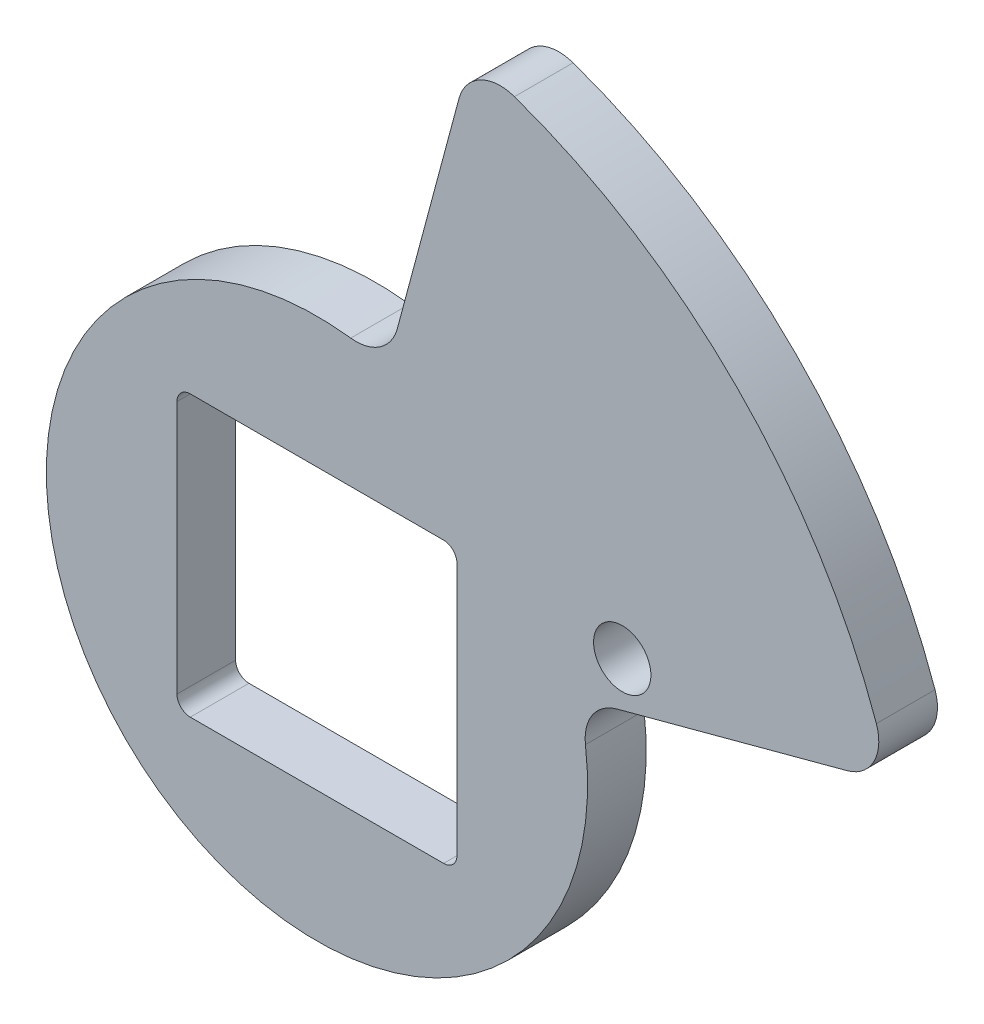
SolidWorks part; units mm, degrees
material "Plain Carbon Steel"
ref_plane "Front Plane" through (0, 0, 0) normal (0, 0, 1) x (1, 0, 0)
ref_plane "Top Plane" through (0, 0, 0) normal (0, 1, 0) x (1, 0, 0)
ref_plane "Right Plane" through (0, 0, 0) normal (1, 0, 0) x (0, 0, -1)
sketch "Lever Plate Profile Sketch" plane through (0, 0, 0) normal (0, 0, 1) x (1, 0, 0)
  line L0 (22.4878, 6.0256) -> (39.7728, 10.6571)
  line L1 (6.0256, 22.4878) -> (10.6571, 39.7728)
  arc A0 (41.9621, 14.8133) -> (14.8133, 41.9621) centre (0, 0) ccw
  arc A1 (2.535, 20.1411) -> (20.1411, 2.535) centre (0, 0) ccw
  arc A2 (14.8133, 41.9621) -> (10.6571, 39.7728) centre (13.7481, 38.9446) ccw
  arc A3 (2.535, 20.1411) -> (6.0256, 22.4878) centre (2.9346, 23.316) ccw
  arc A4 (39.7728, 10.6571) -> (41.9621, 14.8133) centre (38.9446, 13.7481) ccw
  arc A5 (22.4878, 6.0256) -> (20.1411, 2.535) centre (23.316, 2.9346) ccw
  dimension "D1" = 60
  dimension "D2" = 89
  dimension "D3" = 40.6
  dimension "D6" = 3.2
  dimension "D4" = 3.2
  dimension "D5" = 3.2
  dimension "D7" = 3.2
  dimension "D8" = 13.7481
  dimension "D9" = 23.316
  dimension "D10" = 2.9346
extrude "Lever Plate 4.4mm" add sketch "Lever Plate Profile Sketch" along normal blind 4.4
sketch "Square Drive and Pin Hole Sketch" plane through (0, 0, 4.4) normal (0, 0, 1) x (1, 0, 0)
  line L1 (-10.5, 0) -> (-10.5, -9.5)
  line L2 (-9.5, -10.5) -> (9.5, -10.5)
  line L3 (10.5, -9.5) -> (10.5, 9.5)
  line L4 (9.5, 10.5) -> (-9.5, 10.5)
  line L5 (-10.5, 9.5) -> (-10.5, 0)
  arc A1 (-10.5, -9.5) -> (-9.5, -10.5) centre (-9.5, -9.5) ccw
  arc A2 (9.5, -10.5) -> (10.5, -9.5) centre (9.5, -9.5) ccw
  arc A3 (10.5, 9.5) -> (9.5, 10.5) centre (9.5, 9.5) ccw
  arc A4 (-9.5, 10.5) -> (-10.5, 9.5) centre (-9.5, 9.5) ccw
  circle A5 centre (22.9, 9.5) radius 2.15
  point P8 (-10.5, -10.5)
  point P14 (10.5, 10.5)
  point P17 (-10.5, 10.5)
  dimension "D6" = 1
  dimension "D7" = 4.3
  dimension "D1" = 21
  dimension "D2" = 21
  dimension "D3" = 10.5
  dimension "D4" = 10.5
  dimension "D5" = 10.5
  dimension "D8" = 9.5
  dimension "D9" = 22.9
extrude "Square Drive and Pin Hole Cut" cut sketch "Square Drive and Pin Hole Sketch" against normal blind 28.4
